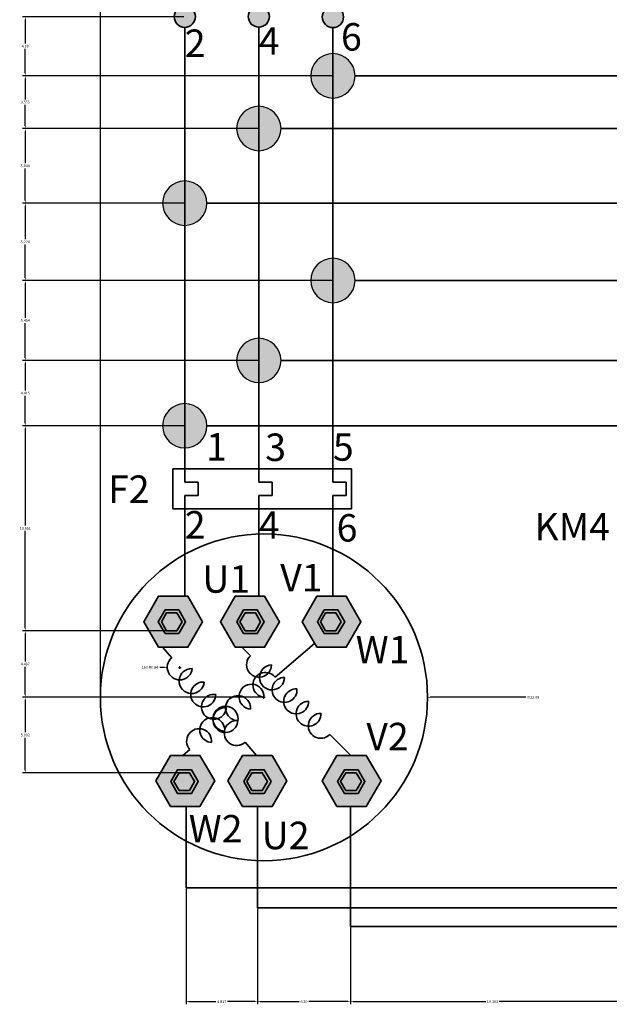
# Model space of a CAD drawing. Units: inches. Extents: x 237 to 313, y 343 to 451.
# Tile 1 of 6: x 237 to 277, y 343 to 410. Entities that reach past the tile are written whole.
import ezdxf

# ---------------------------------------------------------------- set-up
doc = ezdxf.new("R2010")
doc.units = ezdxf.units.IN
doc.header["$MEASUREMENT"] = 0
doc.layers.get('0').update_dxf_attribs({"color": 240})
for name, color, linetype, lineweight in [('A-ANNO-DIMS', 2, 'Continuous', 18), ('E-ANNO-TEXT', 7, 'Continuous', 25), ('E-DEVC', 4, 'Continuous', 35), ('E-MOTR', 3, 'Continuous', 35), ('E-PATT', 8, 'Continuous', 13), ('E-WIRE', 7, 'Continuous', 35), ('E-WIRE-JUNC', 7, 'Continuous', 25)]:
    doc.layers.add(name, color=color, linetype=linetype, lineweight=lineweight)
doc.styles.get("Standard").update_dxf_attribs({"font": 'arial.ttf'})
doc.dimstyles.get("Standard").update_dxf_attribs({"dimtxt": 0.18, "dimasz": 0.18, "dimexe": 0.18, "dimexo": 0.0625, "dimgap": 0.09, "dimtad": 0, "dimtih": 1, "dimtoh": 1, "dimdec": 4, "dimzin": 0, "dimdsep": 46, "dimtxsty": 'Standard', "dimcen": 0.09, "dimadec": 0, "dimazin": 0, "dimtfac": 1, "dimtdec": 4, "dimtofl": 0, "dimtmove": 0, "dimatfit": 3, "dimfxl": 1, "dimtolj": 1, "dimtzin": 0, "dimarcsym": 0})

# ---------------------------------------------------------------- blocks, each defined once
blk = doc.blocks.new('MOTOR-TERMINAL-NUT')
h = blk.add_hatch(color=256)
h.dxf.hatch_style = 1
h.paths.add_polyline_path([(1.386, 1.601), (0.462, 1.601), (0, 0.8), (0.462, 0), (1.386, 0), (1.848, 0.8)])
h.paths.add_polyline_path([(1.607, 0.8), (1.257, 0.195), (0.558, 0.195), (0.209, 0.8), (0.558, 1.406), (1.257, 1.406)], flags=16)
for points in [[(0.462, 0), (1.386, 0), (1.848, 0.8), (1.386, 1.601), (0.462, 1.601), (0, 0.8)], [(0.558, 0.195), (1.257, 0.195), (1.607, 0.8), (1.257, 1.406), (0.558, 1.406), (0.209, 0.8)]]:
    blk.add_lwpolyline(points, close=True)
blk = doc.blocks.new('CONTACTOR-3P-NO')
h = blk.add_hatch(color=256)
h.dxf.hatch_style = 1
h.paths.add_polyline_path([(1.637, 4.965, 1), (1.637, 3.177)])
h.paths.add_polyline_path([(6.637, 4.953, 1), (6.637, 3.166)])
h.paths.add_polyline_path([(11.637, 4.931, 1), (11.637, 3.144)])
h = blk.add_hatch(color=256)
h.dxf.hatch_style = 1
h.paths.add_polyline_path([(2.354, 0.734, 1), (0.92, 0.734, 1)])
h.paths.add_polyline_path([(5.92, 0.749, 1), (7.354, 0.749, 1)])
h.paths.add_polyline_path([(10.92, 0.717, 1), (12.354, 0.717, 1)])
for p, q in [((1.414, 1.415), (0, 3.965)), ((6.423, 1.433), (4.991, 3.965)), ((11.461, 1.412), (9.739, 3.965))]:
    blk.add_line(p, q)
for centre in [(1.637, 0.734), (6.637, 0.749), (11.637, 0.717)]:
    blk.add_circle(centre, 0.717)
for centre in [(1.637, 4.071), (6.637, 4.06), (11.637, 4.037)]:
    blk.add_arc(centre, 0.894, 90, 270)
blk = doc.blocks.new('*D3')
at = {"layer": 'A-ANNO-DIMS', "color": 0, "lineweight": -2, "transparency": 16777216}
for p, q in [((242.3, 363.785), (242.3, 451.078)), ((242.48, 450.898), (274.084, 450.898)), ((306.476, 450.898), (274.872, 450.898)), ((306.656, 382.738), (306.656, 451.078))]:
    blk.add_line(p, q, dxfattribs=at)
at = {"layer": 'A-ANNO-DIMS', "color": 0, "lineweight": 35, "transparency": 16777216}
for points in [[(242.48, 450.928), (242.48, 450.868), (242.3, 450.898)], [(306.476, 450.928), (306.476, 450.868), (306.656, 450.898)]]:
    blk.add_solid(points, dxfattribs=at)
at = {"layer": 'Defpoints', "color": 0, "lineweight": 35, "transparency": 16777216}
for p in [(306.656, 450.898), (306.656, 382.675), (242.3, 363.723)]:
    blk.add_point(p, dxfattribs=at)
at = {"layer": 'A-ANNO-DIMS', "color": 0, "transparency": 16777216, "insert": (274.478, 450.898), "char_height": 0.18, "attachment_point": 5}
blk.add_mtext('\\A1;64.36', dxfattribs=at)
blk = doc.blocks.new('*D4')
at = {"layer": 'A-ANNO-DIMS', "color": 0, "lineweight": -2, "transparency": 16777216}
for p, q in [((258.115, 445.823), (312.65, 445.823)), ((312.47, 445.643), (312.47, 397.21)), ((312.47, 348.414), (312.47, 396.846)), ((289.124, 348.234), (312.65, 348.234))]:
    blk.add_line(p, q, dxfattribs=at)
at = {"layer": 'A-ANNO-DIMS', "color": 0, "lineweight": 35, "transparency": 16777216}
for points in [[(312.44, 445.643), (312.5, 445.643), (312.47, 445.823)], [(312.44, 348.414), (312.5, 348.414), (312.47, 348.234)]]:
    blk.add_solid(points, dxfattribs=at)
at = {"layer": 'Defpoints', "color": 0, "lineweight": 35, "transparency": 16777216}
for p in [(258.052, 445.823), (289.062, 348.234), (312.47, 348.234)]:
    blk.add_point(p, dxfattribs=at)
at = {"layer": 'A-ANNO-DIMS', "color": 0, "transparency": 16777216, "insert": (312.47, 397.028), "char_height": 0.18, "attachment_point": 5}
blk.add_mtext('\\A1;97.59', dxfattribs=at)
blk = doc.blocks.new('*D12')
at = {"layer": 'A-ANNO-DIMS', "color": 0, "lineweight": -2, "transparency": 16777216}
for p, q in [((248.084, 350.796), (248.084, 342.979)), ((252.9, 349.444), (252.9, 342.979)), ((248.264, 343.159), (250.095, 343.159)), ((252.72, 343.159), (250.889, 343.159))]:
    blk.add_line(p, q, dxfattribs=at)
at = {"layer": 'A-ANNO-DIMS', "color": 0, "lineweight": 35, "transparency": 16777216}
for points in [[(248.264, 343.189), (248.264, 343.129), (248.084, 343.159)], [(252.72, 343.189), (252.72, 343.129), (252.9, 343.159)]]:
    blk.add_solid(points, dxfattribs=at)
at = {"layer": 'Defpoints', "color": 0, "lineweight": 35, "transparency": 16777216}
for p in [(248.084, 350.859), (252.9, 349.506), (252.9, 343.159)]:
    blk.add_point(p, dxfattribs=at)
at = {"layer": 'A-ANNO-DIMS', "color": 0, "transparency": 16777216, "insert": (250.492, 343.159), "char_height": 0.18, "attachment_point": 5}
blk.add_mtext('\\A1;4.817', dxfattribs=at)
blk = doc.blocks.new('*D13')
at = {"layer": 'A-ANNO-DIMS', "color": 0, "lineweight": -2, "transparency": 16777216}
for p, q in [((252.9, 349.444), (252.9, 342.979)), ((259.191, 348.171), (259.191, 342.979)), ((253.08, 343.159), (255.721, 343.159)), ((259.011, 343.159), (256.37, 343.159))]:
    blk.add_line(p, q, dxfattribs=at)
at = {"layer": 'A-ANNO-DIMS', "color": 0, "lineweight": 35, "transparency": 16777216}
for points in [[(253.08, 343.189), (253.08, 343.129), (252.9, 343.159)], [(259.011, 343.189), (259.011, 343.129), (259.191, 343.159)]]:
    blk.add_solid(points, dxfattribs=at)
at = {"layer": 'Defpoints', "color": 0, "lineweight": 35, "transparency": 16777216}
for p in [(252.9, 349.506), (259.191, 348.234), (259.191, 343.159)]:
    blk.add_point(p, dxfattribs=at)
at = {"layer": 'A-ANNO-DIMS', "color": 0, "transparency": 16777216, "insert": (256.045, 343.159), "char_height": 0.18, "attachment_point": 5}
blk.add_mtext('\\A1;6.29', dxfattribs=at)
blk = doc.blocks.new('*D14')
at = {"layer": 'A-ANNO-DIMS', "color": 0, "lineweight": -2, "transparency": 16777216}
for p, q in [((278.353, 350.796), (278.353, 342.979)), ((259.191, 348.171), (259.191, 342.979)), ((259.371, 343.159), (268.317, 343.159)), ((278.173, 343.159), (269.227, 343.159))]:
    blk.add_line(p, q, dxfattribs=at)
at = {"layer": 'A-ANNO-DIMS', "color": 0, "lineweight": 35, "transparency": 16777216}
for points in [[(259.371, 343.189), (259.371, 343.129), (259.191, 343.159)], [(278.173, 343.189), (278.173, 343.129), (278.353, 343.159)]]:
    blk.add_solid(points, dxfattribs=at)
at = {"layer": 'Defpoints', "color": 0, "lineweight": 35, "transparency": 16777216}
for p in [(278.353, 350.859), (259.191, 348.234), (278.353, 343.159)]:
    blk.add_point(p, dxfattribs=at)
at = {"layer": 'A-ANNO-DIMS', "color": 0, "transparency": 16777216, "insert": (268.772, 343.159), "char_height": 0.18, "attachment_point": 5}
blk.add_mtext('\\A1;19.163', dxfattribs=at)
blk = doc.blocks.new('*D30')
at = {"layer": 'A-ANNO-DIMS', "color": 0, "lineweight": -2, "transparency": 16777216}
for p, q in [((247.934, 409.714), (237.045, 409.714)), ((237.225, 409.534), (237.225, 407.898)), ((237.225, 405.898), (237.225, 407.534)), ((257.934, 405.718), (237.045, 405.718))]:
    blk.add_line(p, q, dxfattribs=at)
at = {"layer": 'A-ANNO-DIMS', "color": 0, "lineweight": 35, "transparency": 16777216}
for points in [[(237.195, 409.534), (237.255, 409.534), (237.225, 409.714)], [(237.195, 405.898), (237.255, 405.898), (237.225, 405.718)]]:
    blk.add_solid(points, dxfattribs=at)
at = {"layer": 'Defpoints', "color": 0, "lineweight": 35, "transparency": 16777216}
for p in [(247.997, 409.714), (237.225, 405.718), (257.997, 405.718)]:
    blk.add_point(p, dxfattribs=at)
at = {"layer": 'A-ANNO-DIMS', "color": 0, "transparency": 16777216, "insert": (237.225, 407.716), "char_height": 0.18, "attachment_point": 5}
blk.add_mtext('\\A1;4.00', dxfattribs=at)
blk = doc.blocks.new('*D31')
at = {"layer": 'A-ANNO-DIMS', "color": 0, "lineweight": -2, "transparency": 16777216}
for p, q in [((257.934, 405.718), (237.045, 405.718)), ((237.225, 405.538), (237.225, 404.123)), ((237.225, 402.343), (237.225, 403.759)), ((252.934, 402.163), (237.045, 402.163))]:
    blk.add_line(p, q, dxfattribs=at)
at = {"layer": 'A-ANNO-DIMS', "color": 0, "lineweight": 35, "transparency": 16777216}
for points in [[(237.195, 405.538), (237.255, 405.538), (237.225, 405.718)], [(237.195, 402.343), (237.255, 402.343), (237.225, 402.163)]]:
    blk.add_solid(points, dxfattribs=at)
at = {"layer": 'Defpoints', "color": 0, "lineweight": 35, "transparency": 16777216}
for p in [(257.997, 405.718), (237.225, 402.163), (252.997, 402.163)]:
    blk.add_point(p, dxfattribs=at)
at = {"layer": 'A-ANNO-DIMS', "color": 0, "transparency": 16777216, "insert": (237.225, 403.941), "char_height": 0.18, "attachment_point": 5}
blk.add_mtext('\\A1;3.555', dxfattribs=at)
blk = doc.blocks.new('*D32')
at = {"layer": 'A-ANNO-DIMS', "color": 0, "lineweight": -2, "transparency": 16777216}
for p, q in [((252.934, 402.163), (237.045, 402.163)), ((237.225, 401.983), (237.225, 399.821)), ((237.225, 397.295), (237.225, 399.457)), ((247.934, 397.115), (237.045, 397.115))]:
    blk.add_line(p, q, dxfattribs=at)
at = {"layer": 'A-ANNO-DIMS', "color": 0, "lineweight": 35, "transparency": 16777216}
for points in [[(237.195, 401.983), (237.255, 401.983), (237.225, 402.163)], [(237.195, 397.295), (237.255, 397.295), (237.225, 397.115)]]:
    blk.add_solid(points, dxfattribs=at)
at = {"layer": 'Defpoints', "color": 0, "lineweight": 35, "transparency": 16777216}
for p in [(252.997, 402.163), (237.225, 397.115), (247.997, 397.115)]:
    blk.add_point(p, dxfattribs=at)
at = {"layer": 'A-ANNO-DIMS', "color": 0, "transparency": 16777216, "insert": (237.225, 399.639), "char_height": 0.18, "attachment_point": 5}
blk.add_mtext('\\A1;5.048', dxfattribs=at)
blk = doc.blocks.new('*D33')
at = {"layer": 'A-ANNO-DIMS', "color": 0, "lineweight": -2, "transparency": 16777216}
for p, q in [((247.934, 397.115), (237.045, 397.115)), ((237.225, 396.935), (237.225, 394.684)), ((237.225, 392.07), (237.225, 394.321)), ((257.934, 391.89), (237.045, 391.89))]:
    blk.add_line(p, q, dxfattribs=at)
at = {"layer": 'A-ANNO-DIMS', "color": 0, "lineweight": 35, "transparency": 16777216}
for points in [[(237.195, 396.935), (237.255, 396.935), (237.225, 397.115)], [(237.195, 392.07), (237.255, 392.07), (237.225, 391.89)]]:
    blk.add_solid(points, dxfattribs=at)
at = {"layer": 'Defpoints', "color": 0, "lineweight": 35, "transparency": 16777216}
for p in [(247.997, 397.115), (237.225, 391.89), (257.997, 391.89)]:
    blk.add_point(p, dxfattribs=at)
at = {"layer": 'A-ANNO-DIMS', "color": 0, "transparency": 16777216, "insert": (237.225, 394.503), "char_height": 0.18, "attachment_point": 5}
blk.add_mtext('\\A1;5.224', dxfattribs=at)
blk = doc.blocks.new('*D34')
at = {"layer": 'A-ANNO-DIMS', "color": 0, "lineweight": -2, "transparency": 16777216}
for p, q in [((257.934, 391.89), (237.045, 391.89)), ((237.225, 391.71), (237.225, 389.37)), ((237.225, 386.666), (237.225, 389.007)), ((252.934, 386.486), (237.045, 386.486))]:
    blk.add_line(p, q, dxfattribs=at)
at = {"layer": 'A-ANNO-DIMS', "color": 0, "lineweight": 35, "transparency": 16777216}
for points in [[(237.195, 391.71), (237.255, 391.71), (237.225, 391.89)], [(237.195, 386.666), (237.255, 386.666), (237.225, 386.486)]]:
    blk.add_solid(points, dxfattribs=at)
at = {"layer": 'Defpoints', "color": 0, "lineweight": 35, "transparency": 16777216}
for p in [(257.997, 391.89), (237.225, 386.486), (252.997, 386.486)]:
    blk.add_point(p, dxfattribs=at)
at = {"layer": 'A-ANNO-DIMS', "color": 0, "transparency": 16777216, "insert": (237.225, 389.188), "char_height": 0.18, "attachment_point": 5}
blk.add_mtext('\\A1;5.404', dxfattribs=at)
blk = doc.blocks.new('*D35')
at = {"layer": 'A-ANNO-DIMS', "color": 0, "lineweight": -2, "transparency": 16777216}
for p, q in [((252.934, 386.486), (237.045, 386.486)), ((237.225, 386.306), (237.225, 384.461)), ((237.225, 382.251), (237.225, 384.097)), ((247.934, 382.071), (237.045, 382.071))]:
    blk.add_line(p, q, dxfattribs=at)
at = {"layer": 'A-ANNO-DIMS', "color": 0, "lineweight": 35, "transparency": 16777216}
for points in [[(237.195, 386.306), (237.255, 386.306), (237.225, 386.486)], [(237.195, 382.251), (237.255, 382.251), (237.225, 382.071)]]:
    blk.add_solid(points, dxfattribs=at)
at = {"layer": 'Defpoints', "color": 0, "lineweight": 35, "transparency": 16777216}
for p in [(252.997, 386.486), (237.225, 382.071), (247.997, 382.071)]:
    blk.add_point(p, dxfattribs=at)
at = {"layer": 'A-ANNO-DIMS', "color": 0, "transparency": 16777216, "insert": (237.225, 384.279), "char_height": 0.18, "attachment_point": 5}
blk.add_mtext('\\A1;4.415', dxfattribs=at)
blk = doc.blocks.new('*D36')
at = {"layer": 'A-ANNO-DIMS', "color": 0, "lineweight": -2, "transparency": 16777216}
for p, q in [((247.934, 382.071), (237.045, 382.071)), ((237.225, 381.891), (237.225, 375.327)), ((237.225, 368.4), (237.225, 374.963)), ((247.4, 368.22), (237.045, 368.22))]:
    blk.add_line(p, q, dxfattribs=at)
at = {"layer": 'A-ANNO-DIMS', "color": 0, "lineweight": 35, "transparency": 16777216}
for points in [[(237.195, 381.891), (237.255, 381.891), (237.225, 382.071)], [(237.195, 368.4), (237.255, 368.4), (237.225, 368.22)]]:
    blk.add_solid(points, dxfattribs=at)
at = {"layer": 'Defpoints', "color": 0, "lineweight": 35, "transparency": 16777216}
for p in [(247.997, 382.071), (237.225, 368.22), (247.462, 368.22)]:
    blk.add_point(p, dxfattribs=at)
at = {"layer": 'A-ANNO-DIMS', "color": 0, "transparency": 16777216, "insert": (237.225, 375.145), "char_height": 0.18, "attachment_point": 5}
blk.add_mtext('\\A1;13.851', dxfattribs=at)
blk = doc.blocks.new('*D37')
at = {"layer": 'A-ANNO-DIMS', "color": 0, "lineweight": -2, "transparency": 16777216}
for p, q in [((247.4, 368.22), (237.045, 368.22)), ((237.225, 368.04), (237.225, 366.153)), ((237.225, 363.903), (237.225, 365.789)), ((253.282, 363.723), (237.045, 363.723))]:
    blk.add_line(p, q, dxfattribs=at)
at = {"layer": 'A-ANNO-DIMS', "color": 0, "lineweight": 35, "transparency": 16777216}
for points in [[(237.195, 368.04), (237.255, 368.04), (237.225, 368.22)], [(237.195, 363.903), (237.255, 363.903), (237.225, 363.723)]]:
    blk.add_solid(points, dxfattribs=at)
at = {"layer": 'Defpoints', "color": 0, "lineweight": 35, "transparency": 16777216}
for p in [(247.462, 368.22), (237.225, 363.723), (253.344, 363.723)]:
    blk.add_point(p, dxfattribs=at)
at = {"layer": 'A-ANNO-DIMS', "color": 0, "transparency": 16777216, "insert": (237.225, 365.971), "char_height": 0.18, "attachment_point": 5}
blk.add_mtext('\\A1;4.497', dxfattribs=at)
blk = doc.blocks.new('*D38')
at = {"layer": 'A-ANNO-DIMS', "color": 0, "lineweight": -2, "transparency": 16777216}
for p, q in [((253.282, 363.723), (237.045, 363.723)), ((237.225, 363.543), (237.225, 361.359)), ((237.225, 358.811), (237.225, 360.995)), ((248.248, 358.631), (237.045, 358.631))]:
    blk.add_line(p, q, dxfattribs=at)
at = {"layer": 'A-ANNO-DIMS', "color": 0, "lineweight": 35, "transparency": 16777216}
for points in [[(237.195, 363.543), (237.255, 363.543), (237.225, 363.723)], [(237.195, 358.811), (237.255, 358.811), (237.225, 358.631)]]:
    blk.add_solid(points, dxfattribs=at)
at = {"layer": 'Defpoints', "color": 0, "lineweight": 35, "transparency": 16777216}
for p in [(253.344, 363.723), (237.225, 358.631), (248.311, 358.631)]:
    blk.add_point(p, dxfattribs=at)
at = {"layer": 'A-ANNO-DIMS', "color": 0, "transparency": 16777216, "insert": (237.225, 361.177), "char_height": 0.18, "attachment_point": 5}
blk.add_mtext('\\A1;5.092', dxfattribs=at)
blk = doc.blocks.new('*D39')
at = {"layer": 'A-ANNO-DIMS', "color": 0, "lineweight": -2, "transparency": 16777216}
for p, q in [((253.254, 363.723), (253.434, 363.723)), ((253.344, 363.633), (253.344, 363.813)), ((271.015, 363.723), (264.568, 363.723))]:
    blk.add_line(p, q, dxfattribs=at)
at = {"layer": 'A-ANNO-DIMS', "color": 0, "lineweight": 35, "transparency": 16777216}
blk.add_solid([(264.568, 363.753), (264.568, 363.693), (264.388, 363.723)], dxfattribs=at)
at = {"layer": 'Defpoints', "color": 0, "lineweight": 35, "transparency": 16777216}
for p in [(242.3, 363.722), (264.388, 363.723)]:
    blk.add_point(p, dxfattribs=at)
at = {"layer": 'A-ANNO-DIMS', "color": 0, "transparency": 16777216, "insert": (271.506, 363.723), "char_height": 0.18, "attachment_point": 5}
blk.add_mtext('\\A1;∅22.09', dxfattribs=at)
blk = doc.blocks.new('*D43')
at = {"layer": 'A-ANNO-DIMS', "color": 0, "lineweight": -2, "transparency": 16777216}
for p, q in [((246.308, 365.751), (246.633, 365.75)), ((247.566, 365.747), (247.746, 365.747)), ((247.656, 365.657), (247.656, 365.837))]:
    blk.add_line(p, q, dxfattribs=at)
at = {"layer": 'A-ANNO-DIMS', "color": 0, "lineweight": 35, "transparency": 16777216}
blk.add_solid([(246.634, 365.78), (246.633, 365.72), (246.813, 365.75)], dxfattribs=at)
at = {"layer": 'Defpoints', "color": 0, "lineweight": 35, "transparency": 16777216}
for p in [(246.813, 365.75), (247.656, 365.747)]:
    blk.add_point(p, dxfattribs=at)
at = {"layer": 'A-ANNO-DIMS', "color": 0, "transparency": 16777216, "insert": (245.643, 365.751), "char_height": 0.18, "attachment_point": 5}
blk.add_mtext('\\A1;18X R0.84', dxfattribs=at)

msp = doc.modelspace()

# ---------------------------------------------------------------- hatches: boundary and pattern name
at = {"layer": 'E-PATT'}
h = msp.add_hatch(color=256, dxfattribs=at)
h.dxf.hatch_style = 1
h.paths.add_polyline_path([(247.9968, 398.6148), (247.9968, 395.6148, 0.4142136), (249.4968, 397.1148, 0.4142136)])
h.paths.add_polyline_path([(247.9968, 398.6148, 0.4142136), (246.4968, 397.1148, 0.4142136), (247.9968, 395.6148)])
h.paths.add_polyline_path([(254.4968, 402.163, 0.4142136), (252.9968, 403.663), (252.9968, 400.663, 0.4142136)])
h.paths.add_polyline_path([(252.9968, 403.663, 0.4142136), (251.4968, 402.163, 0.4142136), (252.9968, 400.663)])
h.paths.add_polyline_path([(257.9968, 407.2183, 0.4142136), (256.4968, 405.7183, 0.4142136), (257.9968, 404.2183)])
h.paths.add_polyline_path([(259.4968, 405.7183, 0.4142136), (257.9968, 407.2183), (257.9968, 404.2183, 0.4142136)])
h = msp.add_hatch(color=256, dxfattribs=at)
h.dxf.hatch_style = 1
h.paths.add_polyline_path([(249.4968, 382.0712, 1), (246.4968, 382.0712, 1)])
h.paths.add_polyline_path([(254.4968, 386.4864, 0.4142136), (252.9968, 387.9864), (252.9968, 384.9864, 0.4142136)])
h.paths.add_polyline_path([(252.9968, 387.9864, 0.4142136), (251.4968, 386.4864, 0.4142136), (252.9968, 384.9864)])
h.paths.add_polyline_path([(259.4968, 391.8904, 0.4142136), (257.9968, 393.3904), (257.9968, 390.3904, 0.4142136)])
h.paths.add_polyline_path([(257.9968, 393.3904, 0.4142136), (256.4968, 391.8904, 0.4142136), (257.9968, 390.3904)])
h = msp.add_hatch(color=256, dxfattribs=at)
h.dxf.hatch_style = 1
h.paths.add_polyline_path([(245.2238, 368.8253), (246.2186, 367.1023), (248.2082, 367.1023), (249.203, 368.8253), (248.2082, 370.5484), (246.2186, 370.5484)])
h.paths.add_polyline_path([(254.3822, 368.8253), (253.3874, 370.5484), (251.3978, 370.5484), (250.4031, 368.8253), (251.3978, 367.1023), (253.3874, 367.1023)])
h.paths.add_polyline_path([(256.9077, 370.5484), (255.9129, 368.8253), (256.9077, 367.1023), (258.8973, 367.1023), (259.892, 368.8253), (258.8973, 370.5484)])
h.paths.add_polyline_path([(258.2635, 359.8017), (257.2687, 358.0786), (258.2635, 356.3556), (260.2531, 356.3556), (261.2479, 358.0786), (260.2531, 359.8017)])
h.paths.add_polyline_path([(253.8861, 359.8017), (251.8966, 359.8017), (250.9018, 358.0786), (251.8966, 356.3556), (253.8861, 356.3556), (254.8809, 358.0786)])
h.paths.add_polyline_path([(247.0336, 359.8017), (246.0388, 358.0786), (247.0336, 356.3556), (249.0232, 356.3556), (250.018, 358.0786), (249.0232, 359.8017)])

# ---------------------------------------------------------------- linework, layer by layer
at = {"layer": 'E-DEVC'}
for p, q in [((247.9968, 379.1527), (247.9968, 378.2527)), ((252.9968, 379.1527), (252.9968, 378.2527)), ((257.9968, 379.1527), (257.9968, 378.2527)), ((247.9968, 378.2527), (248.8968, 378.2527)), ((248.8968, 378.2527), (248.8968, 377.3527)), ((252.9968, 378.2527), (253.8968, 378.2527)), ((253.8968, 378.2527), (253.8968, 377.3527)), ((257.9968, 378.2527), (258.8968, 378.2527)), ((258.8968, 378.2527), (258.8968, 377.3527)), ((248.8968, 377.3527), (247.9968, 377.3527)), ((247.9968, 377.3527), (247.9968, 376.4527)), ((253.8968, 377.3527), (252.9968, 377.3527)), ((252.9968, 377.3527), (252.9968, 376.4527)), ((258.8968, 377.3527), (257.9968, 377.3527)), ((257.9968, 377.3527), (257.9968, 376.4527))]:
    msp.add_line(p, q, dxfattribs=at)
msp.add_lwpolyline([(247.1871, 379.1527), (259.244, 379.1527), (259.244, 376.4666), (247.1871, 376.4666)], close=True, dxfattribs=at)
at = {"layer": 'E-MOTR'}
for p, q in [((254.0899, 365.0944), (256.7578, 367.3619)), ((247.1158, 366.394), (246.5019, 367.1023)), ((252.4262, 366.5363), (251.8559, 367.1023)), ((252.8301, 359.8017), (252.0655, 360.6837)), ((259.2115, 359.8017), (257.7897, 361.2128)), ((247.8625, 359.8017), (248.3317, 360.2005))]:
    msp.add_line(p, q, dxfattribs=at)
for points in [[(246.2186, 367.1023), (248.2082, 367.1023), (249.203, 368.8253), (248.2082, 370.5484), (246.2186, 370.5484), (245.2238, 368.8253)], [(251.3978, 367.1023), (253.3874, 367.1023), (254.3822, 368.8253), (253.3874, 370.5484), (251.3978, 370.5484), (250.4031, 368.8253)], [(256.9077, 367.1023), (258.8973, 367.1023), (259.892, 368.8253), (258.8973, 370.5484), (256.9077, 370.5484), (255.9129, 368.8253)], [(247.0336, 356.3556), (249.0232, 356.3556), (250.018, 358.0786), (249.0232, 359.8017), (247.0336, 359.8017), (246.0388, 358.0786)], [(251.8966, 356.3556), (253.8861, 356.3556), (254.8809, 358.0786), (253.8861, 359.8017), (251.8966, 359.8017), (250.9018, 358.0786)], [(258.2635, 356.3556), (260.2531, 356.3556), (261.2479, 358.0786), (260.2531, 359.8017), (258.2635, 359.8017), (257.2687, 358.0786)]]:
    msp.add_lwpolyline(points, close=True, dxfattribs=at)
msp.add_circle((253.3442, 363.7227), 11.044, dxfattribs=at)
for centre, start, end in [((247.6562, 365.7472), 129.879868, 354.178802), ((253.0135, 365.9319), 134.175608, 358.474542), ((248.4603, 364.8197), 87.659255, 355.819314), ((253.4379, 364.5603), 39.322546, 263.62148), ((253.8847, 365.0671), 91.954995, 0.115054), ((249.2423, 363.9175), 86.018743, 359.867929), ((254.7321, 364.226), 90.314483, 4.163669), ((252.5025, 363.7654), 357.101932, 265.261991), ((255.5178, 363.4462), 86.265868, 0.746531), ((249.9674, 363.081), 81.970127, 356.450791), ((251.5928, 362.9921), 355.461421, 269.310607), ((256.3559, 362.6144), 89.683006, 1.618864), ((250.7408, 362.1888), 85.387265, 357.323124), ((250.7493, 362.2752), 351.412805, 265.893469), ((257.1808, 361.7956), 88.810673, 316.253929), ((249.8496, 361.5106), 354.829943, 266.765802), ((251.5021, 361.3105), 84.514933, 311.958188), ((248.9639, 360.7578), 353.957611, 221.400866)]:
    msp.add_arc(centre, 0.8428, start, end, dxfattribs=at)
at = {"layer": 'E-WIRE'}
for p, q in [((247.9968, 408.9969), (247.9968, 394.8323)), ((252.9968, 409.0118), (252.9968, 379.1527)), ((257.9968, 408.9797), (257.9968, 379.1527)), ((259.4968, 405.7183), (282.6795, 405.7183)), ((254.4968, 402.163), (287.7431, 402.163)), ((249.4968, 397.1148), (292.7062, 397.1148)), ((247.9968, 394.8323), (247.9968, 382.5536)), ((259.4968, 391.8904), (289.0615, 391.8904)), ((254.4968, 386.4864), (284.0644, 386.4864)), ((247.9968, 382.5536), (247.9968, 379.1527)), ((249.4968, 382.0712), (278.3534, 382.0712)), ((247.9968, 376.4527), (247.9968, 370.5484)), ((252.9968, 376.4527), (252.9968, 370.5484)), ((257.9968, 370.5484), (257.9968, 376.4527)), ((248.0836, 356.3556), (248.0836, 350.8589)), ((252.9002, 356.3556), (252.9002, 349.5062)), ((259.1907, 356.3556), (259.1907, 348.2337)), ((248.0836, 350.8589), (278.3534, 350.8589)), ((252.9002, 349.5062), (284.0644, 349.5062)), ((259.1907, 348.2337), (289.0615, 348.2337))]:
    msp.add_line(p, q, dxfattribs=at)
at = {"layer": 'E-WIRE-JUNC'}
for points in [[(256.4968, 405.7183, 1), (259.4968, 405.7183, 1)], [(251.4968, 402.163, 1), (254.4968, 402.163, 1)], [(246.4968, 397.1148, 1), (249.4968, 397.1148, 1)], [(256.4968, 391.8904, 1), (259.4968, 391.8904, 1)], [(251.4968, 386.4864, 1), (254.4968, 386.4864, 1)], [(246.4968, 382.0712, 1), (249.4968, 382.0712, 1)]]:
    msp.add_lwpolyline(points, format="xyb", close=True, dxfattribs=at)

# ---------------------------------------------------------------- block references
at = {"layer": 'E-DEVC'}
msp.add_blockref('CONTACTOR-3P-NO', (246.36, 408.98), dxfattribs=at)
at = {"layer": 'E-MOTR'}
for p in [(246.205, 368.025), (251.5089, 368.025), (256.948, 368.025), (247.0534, 357.2246), (251.9745, 357.2246), (258.3114, 357.2246)]:
    msp.add_blockref('MOTOR-TERMINAL-NUT', p, dxfattribs=at)

# ---------------------------------------------------------------- texts
at = {"layer": 'E-ANNO-TEXT'}
for s, height, p in [('6', 1.8564, (258.5437, 407.4246)), ('2', 1.8564, (247.9968, 406.996)), ('4', 1.8564, (252.9968, 407.1483)), ('1', 1.8564, (249.4353, 379.7213)), ('3', 1.8564, (253.4269, 379.6922)), ('5', 1.8564, (257.9968, 379.7114)), ('F2', 1.85645, (242.8166, 376.8605)), ('2', 1.8564, (247.9968, 374.4531)), ('4', 1.8564, (252.9968, 374.4395)), ('6', 1.8564, (258.2499, 374.2466)), ('KM4', 1.85645, (271.6096, 374.3223)), ('U1', 1.85645, (249.1827, 370.7904)), ('V1', 1.85645, (254.4396, 370.8762)), ('W1', 1.85645, (259.5419, 366.0208)), ('V2', 1.85645, (260.2531, 360.1418)), ('W2', 1.85645, (248.2642, 353.9164)), ('U2', 1.85645, (253.1893, 353.4606))]:
    msp.add_text(s, height=height, dxfattribs=at).set_placement(p)

# ---------------------------------------------------------------- dimensions: what is measured, and where the dimension line sits
at = {"layer": 'A-ANNO-DIMS'}
for base, p1, p2, override, picture, middle in [((306.6564, 450.8976), (242.3002, 363.7227), (306.6564, 382.675), {"dimdec": 2, "dimlfac": 1, "dimrnd": 0, "dimzin": 0, "dimdsep": 46, "dimlunit": 2}, '*D3', (274.4783, 450.8976)), ((252.9002, 343.1587), (248.0836, 350.8589), (252.9002, 349.5062), {"dimdec": 3, "dimlfac": 1, "dimrnd": 0, "dimzin": 0, "dimdsep": 46, "dimlunit": 2}, '*D12', (250.4919, 343.1587)), ((278.3534, 343.1587), (259.1907, 348.2337), (278.3534, 350.8589), {"dimdec": 3, "dimlfac": 1, "dimrnd": 0, "dimzin": 0, "dimdsep": 46, "dimlunit": 2}, '*D14', (268.7721, 343.1587)), ((259.1907, 343.1587), (252.9002, 349.5062), (259.1907, 348.2337), {"dimdec": 2, "dimlfac": 1, "dimrnd": 0, "dimzin": 0, "dimdsep": 46, "dimlunit": 2}, '*D13', (256.0454, 343.1587))]:
    dim = msp.add_linear_dim(base=base, p1=p1, p2=p2, dimstyle='Standard', override=override, dxfattribs=at)
    dim.commit()
    dim.dimension.update_dxf_attribs({"geometry": picture, "text_midpoint": middle})
for base, p1, p2, override, picture, middle in [((312.4701, 348.2337), (258.0525, 445.8226), (289.0615, 348.2337), {"dimdec": 2, "dimlfac": 1, "dimrnd": 0, "dimzin": 0, "dimdsep": 46, "dimlunit": 2}, '*D4', (312.4701, 397.0282)), ((237.2252, 405.7183), (247.9968, 409.7137), (257.9968, 405.7183), {"dimdec": 2, "dimlfac": 1, "dimrnd": 0, "dimzin": 0, "dimdsep": 46, "dimlunit": 2}, '*D30', (237.2252, 407.716)), ((237.2252, 402.163), (257.9968, 405.7183), (252.9968, 402.163), {"dimdec": 3, "dimlfac": 1, "dimrnd": 0, "dimzin": 0, "dimdsep": 46, "dimlunit": 2}, '*D31', (237.2252, 403.9406)), ((237.2252, 397.1148), (252.9968, 402.163), (247.9968, 397.1148), {"dimdec": 3, "dimlfac": 1, "dimrnd": 0, "dimzin": 0, "dimdsep": 46, "dimlunit": 2}, '*D32', (237.2252, 399.6389)), ((237.2252, 391.8904), (247.9968, 397.1148), (257.9968, 391.8904), {"dimdec": 3, "dimlfac": 1, "dimrnd": 0, "dimzin": 0, "dimdsep": 46, "dimlunit": 2}, '*D33', (237.2252, 394.5026)), ((237.2252, 386.4864), (257.9968, 391.8904), (252.9968, 386.4864), {"dimdec": 3, "dimlfac": 1, "dimrnd": 0, "dimzin": 0, "dimdsep": 46, "dimlunit": 2}, '*D34', (237.2252, 389.1884)), ((237.2252, 382.0712), (252.9968, 386.4864), (247.9968, 382.0712), {"dimdec": 3, "dimlfac": 1, "dimrnd": 0, "dimzin": 0, "dimdsep": 46, "dimlunit": 2}, '*D35', (237.2252, 384.2788)), ((237.2252, 368.2198), (247.9968, 382.0712), (247.4624, 368.2198), {"dimdec": 3, "dimlfac": 1, "dimrnd": 0, "dimzin": 0, "dimdsep": 46, "dimlunit": 2}, '*D36', (237.2252, 375.1455)), ((237.2252, 363.7227), (247.4624, 368.2198), (253.3442, 363.7227), {"dimdec": 3, "dimlfac": 1, "dimrnd": 0, "dimzin": 0, "dimdsep": 46, "dimlunit": 2}, '*D37', (237.2252, 365.9713)), ((237.2252, 358.6306), (253.3442, 363.7227), (248.3108, 358.6306), {"dimdec": 3, "dimlfac": 1, "dimrnd": 0, "dimzin": 0, "dimdsep": 46, "dimlunit": 2}, '*D38', (237.2252, 361.1767))]:
    dim = msp.add_linear_dim(base=base, p1=p1, p2=p2, angle=90, dimstyle='Standard', override=override, dxfattribs=at)
    dim.commit()
    dim.dimension.update_dxf_attribs({"geometry": picture, "text_midpoint": middle})
dim = msp.add_radius_dim(center=(247.6562, 365.7472), mpoint=(246.8134, 365.7499), text='18X <>', dimstyle='Standard', override={"dimdec": 2, "dimlfac": 1, "dimrnd": 0, "dimzin": 0, "dimdsep": 46, "dimlunit": 2}, dxfattribs=at)
dim.commit()
dim.dimension.update_dxf_attribs({"geometry": '*D43', "text_midpoint": (246.3078, 365.7515), "dimtype": 164})
dim = msp.add_diameter_dim_2p(p1=(242.3002, 363.7225), p2=(264.3883, 363.723), dimstyle='Standard', override={"dimdec": 2, "dimlfac": 1, "dimrnd": 0, "dimzin": 0, "dimdsep": 46, "dimlunit": 2}, dxfattribs=at)
dim.commit()
dim.dimension.update_dxf_attribs({"geometry": '*D39', "text_midpoint": (271.0147, 363.7232), "dimtype": 163})

doc.saveas('drawing.dxf')
